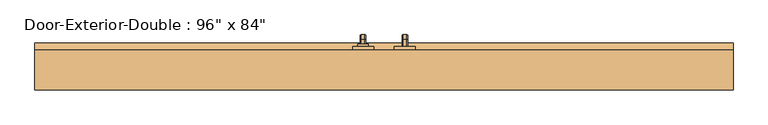
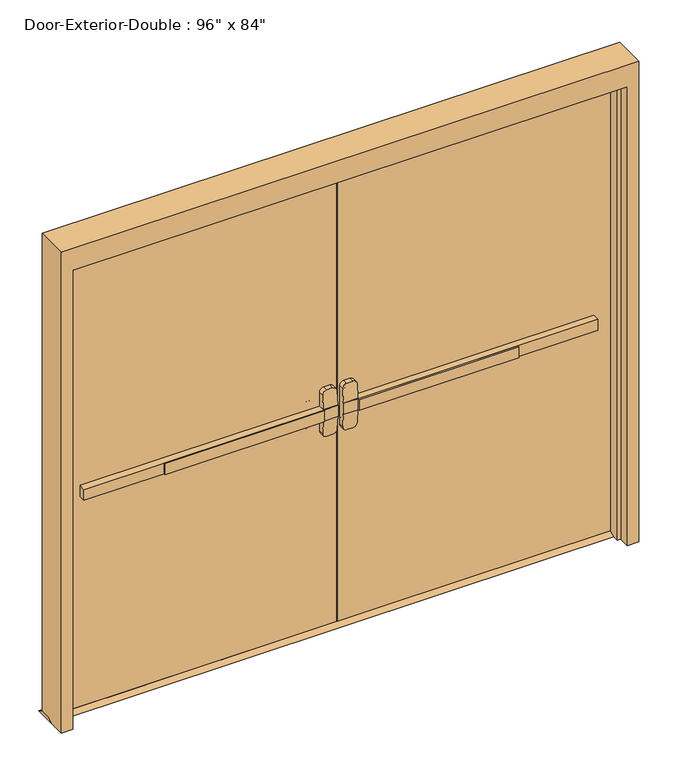
"""IFC4 building model written with IfcOpenShell, lengths in millimetres: door geometry."""

from ifc_helpers import new_model, si_unit, point, frame, frame_2d, origin, place, context, project, spatial, polyline, circle_curve, ellipse_curve, trimmed, segment, composite_curve, outline, extrude, faceted_brep, source, transform, mapped, element, save
from ifc_brep_helpers import plane_surface, cylinder_surface, revolved_surface, advanced_brep


def door_9521ecb0(model_context):
    return source(origin(), model_context, "Body", "SolidModel", [
        extrude(outline(polyline([(-778.9333333, 0.0), (-778.9333333, 6.35), (-76.2, 6.35), (-76.2, 0.0), (-778.9333333, 0.0)])), frame((0.0, 0.0, 990.6), z_axis=(0.0, 0.0, 1.0), x_axis=(1.0, 0.0, 0.0)), (0.0, 0.0, 1.0), 50.8),
        advanced_brep(
        [(-12.7, 6.35, 1041.4), (-76.2, 6.35, 1041.4), (-1130.3, 6.35, 1041.4), (-1130.3, 6.35, 990.6), (-76.2, 6.35, 990.6), (-12.7, 6.35, 990.6), (-1130.3, 38.1, 1041.4), (-76.2, 38.1, 1041.4), (-76.2, 38.1, 1104.9), (-57.15, 38.1, 1123.95), (-31.75, 38.1, 1123.95), (-12.7, 38.1, 1104.9), (-12.7, 38.1, 927.1), (-31.75, 38.1, 908.05), (-57.15, 38.1, 908.05), (-76.2, 38.1, 927.1), (-76.2, 38.1, 990.6), (-1130.3, 38.1, 990.6), (-12.7, 9.5252467, 1041.4), (-76.2, 9.5252467, 1041.4), (-12.7, 9.5252467, 990.6), (-12.7, 14.5354269, 927.1), (-12.7, 14.5354269, 1104.9), (-76.2, 9.5252467, 990.6), (-76.2, 14.5354269, 1104.9), (-76.2, 14.5354269, 927.1), (-57.15, 16.038481, 1123.95), (-31.75, 16.038481, 1123.95), (-31.75, 16.038481, 908.05), (-57.15, 16.038481, 908.05)],
        [
            (0, 1),
            (1, 2),
            (2, 3),
            (3, 4),
            (4, 5),
            (5, 0),
            (6, 7),
            (7, 8),
            (8, 9, circle_curve(frame((-57.15, 38.1, 1104.9), z_axis=(0.0, 1.0, 0.0), x_axis=(-1.0, 0.0, 0.0)), 19.05)),
            (9, 10),
            (10, 11, circle_curve(frame((-31.75, 38.1, 1104.9), z_axis=(0.0, 1.0, 0.0), x_axis=(-1.0, 0.0, 0.0)), 19.05)),
            (11, 12),
            (12, 13, circle_curve(frame((-31.75, 38.1, 927.1), z_axis=(0.0, 1.0, 0.0), x_axis=(-1.0, 0.0, 0.0)), 19.05)),
            (13, 14),
            (14, 15, circle_curve(frame((-57.15, 38.1, 927.1), z_axis=(0.0, 1.0, 0.0), x_axis=(-1.0, 0.0, 0.0)), 19.05)),
            (15, 16),
            (16, 17),
            (17, 6),
            (0, 18),
            (18, 19),
            (19, 7),
            (6, 2),
            (5, 20),
            (20, 21),
            (21, 12),
            (11, 22),
            (22, 18),
            (16, 23),
            (23, 20),
            (3, 17),
            (19, 24),
            (24, 8),
            (15, 25),
            (25, 23),
            (9, 26),
            (26, 27),
            (27, 10),
            (13, 28),
            (28, 29),
            (29, 14),
            (29, 25, ellipse_curve(frame((-57.15, 14.5354269, 927.1), z_axis=(0.0, 0.9969018152893365, 0.07865602756830282), x_axis=(0.0, -0.07865602756830208, 0.9969018152893365)), 19.1092038, 19.05)),
            (24, 26, ellipse_curve(frame((-57.15, 14.5354269, 1104.9), z_axis=(0.0, 0.9969018152893376, -0.07865602756828934), x_axis=(0.0, -0.078656027568288, -0.9969018152893377)), 19.1092038, 19.05)),
            (27, 22, ellipse_curve(frame((-31.75, 14.5354269, 1104.9), z_axis=(0.0, 0.9969018152893376, -0.07865602756828934), x_axis=(0.0, -0.078656027568288, -0.9969018152893377)), 19.1092038, 19.05)),
            (21, 28, ellipse_curve(frame((-31.75, 14.5354269, 927.1), z_axis=(0.0, 0.9969018152893365, 0.07865602756830282), x_axis=(0.0, -0.07865602756830208, 0.9969018152893365)), 19.1092038, 19.05)),
        ],
        [
            plane_surface(frame((-12.7, 6.35, 1041.4), z_axis=(0.0, -1.0, 0.0), x_axis=(1.0, 0.0, 0.0))),
            plane_surface(frame((-12.7, 38.1, 1041.4), z_axis=(0.0, 1.0, 0.0), x_axis=(-1.0, 0.0, 0.0))),
            plane_surface(frame((-1130.3, 6.35, 1041.4), z_axis=(0.0, 0.0, 1.0), x_axis=(0.0, 1.0, 0.0))),
            plane_surface(frame((-12.7, 6.35, 1041.4), z_axis=(1.0, 0.0, 0.0), x_axis=(0.0, 1.0, 0.0))),
            plane_surface(frame((-12.7, 6.35, 990.6), z_axis=(0.0, 0.0, -1.0), x_axis=(0.0, 1.0, 0.0))),
            plane_surface(frame((-1130.3, 6.35, 990.6), z_axis=(-1.0, 0.0, 0.0), x_axis=(0.0, 1.0, 0.0))),
            plane_surface(frame((-76.2, 9.5252467, 927.1), z_axis=(-1.0, 0.0, 0.0), x_axis=(0.0, 1.0, 0.0))),
            plane_surface(frame((-57.15, 9.5252467, 1123.95), z_axis=(0.0, 0.0, 1.0), x_axis=(0.0, 1.0, 0.0))),
            plane_surface(frame((-31.75, 9.5252467, 908.05), z_axis=(0.0, 0.0, -1.0), x_axis=(0.0, 1.0, 0.0))),
            cylinder_surface(frame((-57.15, 38.1, 927.1), z_axis=(0.0, -1.0, 0.0), x_axis=(-1.0, 0.0, 0.0)), 19.05),
            cylinder_surface(frame((-57.15, 38.1, 1104.9), z_axis=(0.0, -1.0, 0.0), x_axis=(-1.0, 0.0, 0.0)), 19.05),
            cylinder_surface(frame((-31.75, 38.1, 1104.9), z_axis=(0.0, -1.0, 0.0), x_axis=(-1.0, 0.0, 0.0)), 19.05),
            cylinder_surface(frame((-31.75, 38.1, 927.1), z_axis=(0.0, -1.0, 0.0), x_axis=(-1.0, 0.0, 0.0)), 19.05),
            plane_surface(frame((-76.2, 9.5252467, 1041.4), z_axis=(0.0, -0.9969018152893376, 0.07865602756828934), x_axis=(1.0, 0.0, 0.0))),
            plane_surface(frame((-76.2, 16.038481, 908.05), z_axis=(0.0, -0.9969018152893365, -0.07865602756830282), x_axis=(1.0, 0.0, 0.0))),
        ],
        [
            (0, [[1, 2, 3, 4, 5, 6]]),
            (1, [[7, 8, 9, 10, 11, 12, 13, 14, 15, 16, 17, 18]]),
            (2, [[-2, -1, 19, 20, 21, -7, 22]]),
            (3, [[23, 24, 25, -12, 26, 27, -19, -6]]),
            (4, [[-17, 28, 29, -23, -5, -4, 30]]),
            (5, [[-22, -18, -30, -3]]),
            (6, [[-21, 31, 32, -8]]),
            (6, [[33, 34, -28, -16]]),
            (7, [[35, 36, 37, -10]]),
            (8, [[38, 39, 40, -14]]),
            (9, [[-40, 41, -33, -15]]),
            (10, [[-32, 42, -35, -9]]),
            (11, [[-37, 43, -26, -11]]),
            (12, [[-25, 44, -38, -13]]),
            (13, [[-27, -43, -36, -42, -31, -20]]),
            (14, [[-29, -34, -41, -39, -44, -24]]),
        ],
    ),
        extrude(outline(polyline([(82.55, 12.7), (107.95, 0.0), (12.7, 0.0), (38.1, 12.7), (82.55, 12.7)])), frame((-1270.0, 0.0, 0.0), z_axis=(1.0, 0.0, 0.0), x_axis=(0.0, 1.0, 0.0)), (0.0, 0.0, 1.0), 2540.0),
        extrude(outline(polyline([(778.9333333, 0.0), (76.2, 0.0), (76.2, 6.35), (778.9333333, 6.35), (778.9333333, 0.0)])), frame((0.0, 0.0, 990.6), z_axis=(0.0, 0.0, 1.0), x_axis=(1.0, 0.0, 0.0)), (0.0, 0.0, 1.0), 50.8),
        advanced_brep(
        [(12.7, 6.35, 1041.4), (12.7, 6.35, 990.6), (76.2, 6.35, 990.6), (1130.3, 6.35, 990.6), (1130.3, 6.35, 1041.4), (76.2, 6.35, 1041.4), (1130.3, 38.1, 1041.4), (1130.3, 38.1, 990.6), (76.2, 38.1, 990.6), (76.2, 38.1, 927.1), (57.15, 38.1, 908.05), (31.75, 38.1, 908.05), (12.7, 38.1, 927.1), (12.7, 38.1, 1104.9), (31.75, 38.1, 1123.95), (57.15, 38.1, 1123.95), (76.2, 38.1, 1104.9), (76.2, 38.1, 1041.4), (76.2, 9.5252467, 1041.4), (12.7, 9.5252467, 1041.4), (12.7, 14.5354269, 1104.9), (12.7, 14.5354269, 927.1), (12.7, 9.5252467, 990.6), (76.2, 9.5252467, 990.6), (76.2, 14.5354269, 927.1), (76.2, 14.5354269, 1104.9), (31.75, 16.038481, 1123.95), (57.15, 16.038481, 1123.95), (57.15, 16.038481, 908.05), (31.75, 16.038481, 908.05)],
        [
            (0, 1),
            (1, 2),
            (2, 3),
            (3, 4),
            (4, 5),
            (5, 0),
            (6, 7),
            (7, 8),
            (8, 9),
            (9, 10, circle_curve(frame((57.15, 38.1, 927.1), z_axis=(0.0, 1.0, 0.0), x_axis=(1.0, 0.0, 0.0)), 19.05)),
            (10, 11),
            (11, 12, circle_curve(frame((31.75, 38.1, 927.1), z_axis=(0.0, 1.0, 0.0), x_axis=(1.0, 0.0, 0.0)), 19.05)),
            (12, 13),
            (13, 14, circle_curve(frame((31.75, 38.1, 1104.9), z_axis=(0.0, 1.0, 0.0), x_axis=(1.0, 0.0, 0.0)), 19.05)),
            (14, 15),
            (15, 16, circle_curve(frame((57.15, 38.1, 1104.9), z_axis=(0.0, 1.0, 0.0), x_axis=(1.0, 0.0, 0.0)), 19.05)),
            (16, 17),
            (17, 6),
            (4, 6),
            (17, 18),
            (18, 19),
            (19, 0),
            (19, 20),
            (20, 13),
            (12, 21),
            (21, 22),
            (22, 1),
            (7, 3),
            (22, 23),
            (23, 8),
            (23, 24),
            (24, 9),
            (16, 25),
            (25, 18),
            (14, 26),
            (26, 27),
            (27, 15),
            (10, 28),
            (28, 29),
            (29, 11),
            (24, 28, ellipse_curve(frame((57.15, 14.5354269, 927.1), z_axis=(0.0, 0.9969018152893365, 0.07865602756830282), x_axis=(0.0, -0.07865602756830208, 0.9969018152893365)), 19.1092038, 19.05)),
            (27, 25, ellipse_curve(frame((57.15, 14.5354269, 1104.9), z_axis=(0.0, 0.9969018152893376, -0.07865602756828934), x_axis=(0.0, -0.078656027568288, -0.9969018152893377)), 19.1092038, 19.05)),
            (20, 26, ellipse_curve(frame((31.75, 14.5354269, 1104.9), z_axis=(0.0, 0.9969018152893376, -0.07865602756828934), x_axis=(0.0, -0.078656027568288, -0.9969018152893377)), 19.1092038, 19.05)),
            (29, 21, ellipse_curve(frame((31.75, 14.5354269, 927.1), z_axis=(0.0, 0.9969018152893365, 0.07865602756830282), x_axis=(0.0, -0.07865602756830208, 0.9969018152893365)), 19.1092038, 19.05)),
        ],
        [
            plane_surface(frame((12.7, 6.35, 1041.4), z_axis=(0.0, -1.0, 0.0), x_axis=(-1.0, 0.0, 0.0))),
            plane_surface(frame((12.7, 38.1, 1041.4), z_axis=(0.0, 1.0, 0.0), x_axis=(1.0, 0.0, 0.0))),
            plane_surface(frame((1130.3, 6.35, 1041.4), z_axis=(0.0, 0.0, 1.0), x_axis=(0.0, 1.0, 0.0))),
            plane_surface(frame((12.7, 6.35, 1041.4), z_axis=(-1.0, 0.0, 0.0), x_axis=(0.0, 1.0, 0.0))),
            plane_surface(frame((12.7, 6.35, 990.6), z_axis=(0.0, 0.0, -1.0), x_axis=(0.0, 1.0, 0.0))),
            plane_surface(frame((1130.3, 6.35, 990.6), z_axis=(1.0, 0.0, 0.0), x_axis=(0.0, 1.0, 0.0))),
            plane_surface(frame((76.2, 9.5252467, 927.1), z_axis=(1.0, 0.0, 0.0), x_axis=(0.0, 1.0, 0.0))),
            plane_surface(frame((57.15, 9.5252467, 1123.95), z_axis=(0.0, 0.0, 1.0), x_axis=(0.0, 1.0, 0.0))),
            plane_surface(frame((31.75, 9.5252467, 908.05), z_axis=(0.0, 0.0, -1.0), x_axis=(0.0, 1.0, 0.0))),
            cylinder_surface(frame((57.15, 38.1, 927.1), z_axis=(0.0, -1.0, 0.0), x_axis=(1.0, 0.0, 0.0)), 19.05),
            cylinder_surface(frame((57.15, 38.1, 1104.9), z_axis=(0.0, -1.0, 0.0), x_axis=(1.0, 0.0, 0.0)), 19.05),
            cylinder_surface(frame((31.75, 38.1, 1104.9), z_axis=(0.0, -1.0, 0.0), x_axis=(1.0, 0.0, 0.0)), 19.05),
            cylinder_surface(frame((31.75, 38.1, 927.1), z_axis=(0.0, -1.0, 0.0), x_axis=(1.0, 0.0, 0.0)), 19.05),
            plane_surface(frame((76.2, 9.5252467, 1041.4), z_axis=(0.0, -0.9969018152893376, 0.07865602756828934), x_axis=(-1.0, 0.0, 0.0))),
            plane_surface(frame((76.2, 16.038481, 908.05), z_axis=(0.0, -0.9969018152893365, -0.07865602756830282), x_axis=(-1.0, 0.0, 0.0))),
        ],
        [
            (0, [[1, 2, 3, 4, 5, 6]]),
            (1, [[7, 8, 9, 10, 11, 12, 13, 14, 15, 16, 17, 18]]),
            (2, [[19, -18, 20, 21, 22, -6, -5]]),
            (3, [[-1, -22, 23, 24, -13, 25, 26, 27]]),
            (4, [[28, -3, -2, -27, 29, 30, -8]]),
            (5, [[-4, -28, -7, -19]]),
            (6, [[-9, -30, 31, 32]]),
            (6, [[-17, 33, 34, -20]]),
            (7, [[-15, 35, 36, 37]]),
            (8, [[-11, 38, 39, 40]]),
            (9, [[-10, -32, 41, -38]]),
            (10, [[-16, -37, 42, -33]]),
            (11, [[-14, -24, 43, -35]]),
            (12, [[-12, -40, 44, -25]]),
            (13, [[-21, -34, -42, -36, -43, -23]]),
            (14, [[-26, -44, -39, -41, -31, -29]]),
        ],
    ),
        advanced_brep(
        [(66.2, 95.25, 1017.190625), (66.2, 95.25, 1014.809375), (69.771875, 95.25, 1011.2375), (82.6284594, 95.25, 1011.2375), (86.2, 95.25, 1014.8090406), (86.2, 95.25, 1017.190625), (82.628125, 95.25, 1020.7625), (69.771875, 95.25, 1020.7625), (66.2, 95.25, 887.809375), (69.771875, 95.25, 884.2375), (82.628125, 95.25, 884.2375), (86.2, 95.25, 887.809375), (86.2, 95.25, 890.1909594), (82.6284594, 95.25, 893.7625), (69.771875, 95.25, 893.7625), (66.2, 95.25, 890.190625), (66.2, 120.65, 1017.190625), (66.2, 134.540625, 1003.3), (66.2, 134.540625, 901.7), (66.2, 120.65, 887.809375), (66.2, 120.65, 890.190625), (66.2, 132.159375, 901.7), (66.2, 132.159375, 1003.3), (66.2, 120.65, 1014.809375), (69.771875, 120.65, 1011.2375), (82.6284594, 120.65, 1011.2375), (86.2, 120.65, 1014.8090406), (86.2, 132.1590406, 1003.3), (86.2, 132.1590406, 901.7), (86.2, 120.65, 890.1909594), (86.2, 120.65, 887.809375), (86.2, 134.540625, 901.7), (86.2, 134.540625, 1003.3), (86.2, 120.65, 1017.190625), (82.628125, 120.65, 1020.7625), (69.771875, 120.65, 1020.7625), (69.771875, 128.5875, 1003.3), (82.6284594, 128.5875, 1003.3), (82.628125, 138.1125, 1003.3), (69.771875, 138.1125, 1003.3), (69.771875, 128.5875, 901.7), (82.6284594, 128.5875, 901.7), (82.628125, 138.1125, 901.7), (69.771875, 138.1125, 901.7), (69.771875, 120.65, 893.7625), (82.6284594, 120.65, 893.7625), (82.628125, 120.65, 884.2375), (69.771875, 120.65, 884.2375)],
        [
            (0, 1),
            (1, 2, circle_curve(frame((69.771875, 95.25, 1014.809375), z_axis=(0.0, -1.0, 0.0), x_axis=(0.0, 0.0, 1.0)), 3.571875)),
            (2, 3),
            (3, 4, circle_curve(frame((82.6284594, 95.25, 1014.8090406), z_axis=(0.0, -1.0, 0.0), x_axis=(0.0, 0.0, 1.0)), 3.5715406)),
            (4, 5),
            (5, 6, circle_curve(frame((82.628125, 95.25, 1017.190625), z_axis=(0.0, -1.0, 0.0), x_axis=(0.0, 0.0, 1.0)), 3.571875)),
            (6, 7),
            (7, 0, circle_curve(frame((69.771875, 95.25, 1017.190625), z_axis=(0.0, -1.0, 0.0), x_axis=(0.0, 0.0, 1.0)), 3.571875)),
            (8, 9, circle_curve(frame((69.771875, 95.25, 887.809375), z_axis=(0.0, -1.0, 0.0), x_axis=(0.0, 0.0, -1.0)), 3.571875)),
            (9, 10),
            (10, 11, circle_curve(frame((82.628125, 95.25, 887.809375), z_axis=(0.0, -1.0, 0.0), x_axis=(0.0, 0.0, -1.0)), 3.571875)),
            (11, 12),
            (12, 13, circle_curve(frame((82.6284594, 95.25, 890.1909594), z_axis=(0.0, -1.0, 0.0), x_axis=(0.0, 0.0, -1.0)), 3.5715406)),
            (13, 14),
            (14, 15, circle_curve(frame((69.771875, 95.25, 890.190625), z_axis=(0.0, -1.0, 0.0), x_axis=(0.0, 0.0, -1.0)), 3.571875)),
            (15, 8),
            (0, 16),
            (16, 17, circle_curve(frame((66.2, 120.65, 1003.3), z_axis=(-1.0, 0.0, 0.0), x_axis=(0.0, 0.0, 1.0)), 13.890625)),
            (17, 18),
            (18, 19, circle_curve(frame((66.2, 120.65, 901.7), z_axis=(-1.0, 0.0, 0.0), x_axis=(0.0, 1.0, 0.0)), 13.890625)),
            (19, 8),
            (15, 20),
            (20, 21, circle_curve(frame((66.2, 120.65, 901.7), z_axis=(1.0, 0.0, 0.0), x_axis=(0.0, 1.0, 0.0)), 11.509375)),
            (21, 22),
            (22, 23, circle_curve(frame((66.2, 120.65, 1003.3), z_axis=(1.0, 0.0, 0.0), x_axis=(0.0, 0.0, 1.0)), 11.509375)),
            (23, 1),
            (23, 24, circle_curve(frame((69.771875, 120.65, 1014.809375), z_axis=(0.0, -1.0, 0.0), x_axis=(0.0, 0.0, 1.0)), 3.571875)),
            (24, 2),
            (24, 25),
            (25, 3),
            (25, 26, circle_curve(frame((82.6284594, 120.65, 1014.8090406), z_axis=(0.0, -1.0, 0.0), x_axis=(0.0, 0.0, 1.0)), 3.5715406)),
            (26, 4),
            (26, 27, circle_curve(frame((86.2, 120.65, 1003.3), z_axis=(-1.0, 0.0, 0.0), x_axis=(0.0, 0.0, 1.0)), 11.5090406)),
            (27, 28),
            (28, 29, circle_curve(frame((86.2, 120.65, 901.7), z_axis=(-1.0, 0.0, 0.0), x_axis=(0.0, 1.0, 0.0)), 11.5090406)),
            (29, 12),
            (11, 30),
            (30, 31, circle_curve(frame((86.2, 120.65, 901.7), z_axis=(1.0, 0.0, 0.0), x_axis=(0.0, 1.0, 0.0)), 13.890625)),
            (31, 32),
            (32, 33, circle_curve(frame((86.2, 120.65, 1003.3), z_axis=(1.0, 0.0, 0.0), x_axis=(0.0, 0.0, 1.0)), 13.890625)),
            (33, 5),
            (33, 34, circle_curve(frame((82.628125, 120.65, 1017.190625), z_axis=(0.0, -1.0, 0.0), x_axis=(0.0, 0.0, 1.0)), 3.571875)),
            (34, 6),
            (34, 35),
            (35, 7),
            (35, 16, circle_curve(frame((69.771875, 120.65, 1017.190625), z_axis=(0.0, -1.0, 0.0), x_axis=(0.0, 0.0, 1.0)), 3.571875)),
            (36, 24, circle_curve(frame((69.771875, 120.65, 1003.3), z_axis=(1.0, 0.0, 0.0), x_axis=(0.0, 0.0, 1.0)), 7.9375)),
            (22, 36, circle_curve(frame((69.771875, 132.159375, 1003.3), z_axis=(0.0, 0.0, 1.0), x_axis=(0.0, 1.0, 0.0)), 3.571875)),
            (37, 25, circle_curve(frame((82.6284594, 120.65, 1003.3), z_axis=(1.0, 0.0, 0.0), x_axis=(0.0, 0.0, 1.0)), 7.9375)),
            (36, 37),
            (37, 27, circle_curve(frame((82.6284594, 132.1590406, 1003.3), z_axis=(0.0, 0.0, 1.0), x_axis=(0.0, 1.0, 0.0)), 3.5715406)),
            (38, 34, circle_curve(frame((82.628125, 120.65, 1003.3), z_axis=(1.0, 0.0, 0.0), x_axis=(0.0, 0.0, 1.0)), 17.4625)),
            (32, 38, circle_curve(frame((82.628125, 134.540625, 1003.3), z_axis=(0.0, 0.0, 1.0), x_axis=(0.0, 1.0, 0.0)), 3.571875)),
            (39, 35, circle_curve(frame((69.771875, 120.65, 1003.3), z_axis=(1.0, 0.0, 0.0), x_axis=(0.0, 0.0, 1.0)), 17.4625)),
            (38, 39),
            (39, 17, circle_curve(frame((69.771875, 134.540625, 1003.3), z_axis=(0.0, 0.0, 1.0), x_axis=(0.0, 1.0, 0.0)), 3.571875)),
            (21, 40, circle_curve(frame((69.771875, 132.159375, 901.7), z_axis=(0.0, 0.0, 1.0), x_axis=(0.0, 1.0, 0.0)), 3.571875)),
            (40, 36),
            (40, 41),
            (41, 37),
            (41, 28, circle_curve(frame((82.6284594, 132.1590406, 901.7), z_axis=(0.0, 0.0, 1.0), x_axis=(0.0, 1.0, 0.0)), 3.5715406)),
            (31, 42, circle_curve(frame((82.628125, 134.540625, 901.7), z_axis=(0.0, 0.0, 1.0), x_axis=(0.0, 1.0, 0.0)), 3.571875)),
            (42, 38),
            (42, 43),
            (43, 39),
            (43, 18, circle_curve(frame((69.771875, 134.540625, 901.7), z_axis=(0.0, 0.0, 1.0), x_axis=(0.0, 1.0, 0.0)), 3.571875)),
            (44, 40, circle_curve(frame((69.771875, 120.65, 901.7), z_axis=(1.0, 0.0, 0.0), x_axis=(0.0, 1.0, 0.0)), 7.9375)),
            (20, 44, circle_curve(frame((69.771875, 120.65, 890.190625), z_axis=(0.0, 1.0, 0.0), x_axis=(0.0, 0.0, -1.0)), 3.571875)),
            (45, 41, circle_curve(frame((82.6284594, 120.65, 901.7), z_axis=(1.0, 0.0, 0.0), x_axis=(0.0, 1.0, 0.0)), 7.9375)),
            (44, 45),
            (45, 29, circle_curve(frame((82.6284594, 120.65, 890.1909594), z_axis=(0.0, 1.0, 0.0), x_axis=(0.0, 0.0, -1.0)), 3.5715406)),
            (46, 42, circle_curve(frame((82.628125, 120.65, 901.7), z_axis=(1.0, 0.0, 0.0), x_axis=(0.0, 1.0, 0.0)), 17.4625)),
            (30, 46, circle_curve(frame((82.628125, 120.65, 887.809375), z_axis=(0.0, 1.0, 0.0), x_axis=(0.0, 0.0, -1.0)), 3.571875)),
            (47, 43, circle_curve(frame((69.771875, 120.65, 901.7), z_axis=(1.0, 0.0, 0.0), x_axis=(0.0, 1.0, 0.0)), 17.4625)),
            (46, 47),
            (47, 19, circle_curve(frame((69.771875, 120.65, 887.809375), z_axis=(0.0, 1.0, 0.0), x_axis=(0.0, 0.0, -1.0)), 3.571875)),
            (14, 44),
            (13, 45),
            (10, 46),
            (9, 47),
        ],
        [
            plane_surface(frame((76.2, 95.25, 1016.0), z_axis=(0.0, -1.0, 0.0), x_axis=(1.0, 0.0, 0.0))),
            plane_surface(frame((76.2, 95.25, 889.0), z_axis=(0.0, -1.0, 0.0), x_axis=(1.0, 0.0, 0.0))),
            plane_surface(frame((66.2, 95.25, 1017.190625), z_axis=(-1.0, 0.0, 0.0), x_axis=(0.0, 1.0, 0.0))),
            cylinder_surface(frame((69.771875, 95.25, 1014.809375), z_axis=(0.0, -1.0, 0.0), x_axis=(0.0, 0.0, 1.0)), 3.571875),
            plane_surface(frame((69.771875, 95.25, 1011.2375), z_axis=(0.0, 0.0, -1.0), x_axis=(0.0, 1.0, 0.0))),
            cylinder_surface(frame((82.6284594, 95.25, 1014.8090406), z_axis=(0.0, -1.0, 0.0), x_axis=(0.0, 0.0, 1.0)), 3.5715406),
            plane_surface(frame((86.2, 95.25, 1014.8090406), z_axis=(1.0, 0.0, 0.0), x_axis=(0.0, 1.0, 0.0))),
            cylinder_surface(frame((82.628125, 95.25, 1017.190625), z_axis=(0.0, -1.0, 0.0), x_axis=(0.0, 0.0, 1.0)), 3.571875),
            plane_surface(frame((82.628125, 95.25, 1020.7625), z_axis=(0.0, 0.0, 1.0), x_axis=(0.0, 1.0, 0.0))),
            cylinder_surface(frame((69.771875, 95.25, 1017.190625), z_axis=(0.0, -1.0, 0.0), x_axis=(0.0, 0.0, 1.0)), 3.571875),
            revolved_surface(trimmed(ellipse_curve(frame((69.771875, 120.65, 1014.809375), z_axis=(0.0, -1.0, 0.0), x_axis=(0.0, 0.0, 1.0)), 3.571875, 3.571875), [point((66.2, 120.65, 1014.809375))], [point((69.771875, 120.65, 1011.2375))], True, "CARTESIAN"), (76.2, 120.65, 1003.3), (-1.0, 0.0, 0.0)),
            revolved_surface(polyline([(69.771875, 120.65, 1011.2375), (82.6284594, 120.65, 1011.2375)]), (76.2, 120.65, 1003.3), (-1.0, 0.0, 0.0)),
            revolved_surface(trimmed(ellipse_curve(frame((82.6284594, 120.65, 1014.8090406), z_axis=(0.0, -1.0, 0.0), x_axis=(0.0, 0.0, 1.0)), 3.5715406, 3.5715406), [point((82.6284594, 120.65, 1011.2375))], [point((86.2, 120.65, 1014.8090406))], True, "CARTESIAN"), (76.2, 120.65, 1003.3), (-1.0, 0.0, 0.0)),
            revolved_surface(trimmed(ellipse_curve(frame((82.628125, 120.65, 1017.190625), z_axis=(0.0, -1.0, 0.0), x_axis=(0.0, 0.0, 1.0)), 3.571875, 3.571875), [point((86.2, 120.65, 1017.190625))], [point((82.628125, 120.65, 1020.7625))], True, "CARTESIAN"), (76.2, 120.65, 1003.3), (-1.0, 0.0, 0.0)),
            cylinder_surface(frame((76.2, 120.65, 1003.3), z_axis=(-1.0, 0.0, 0.0), x_axis=(0.0, 0.0, 1.0)), 17.4625),
            revolved_surface(trimmed(ellipse_curve(frame((69.771875, 120.65, 1017.190625), z_axis=(0.0, -1.0, 0.0), x_axis=(0.0, 0.0, 1.0)), 3.571875, 3.571875), [point((69.771875, 120.65, 1020.7625))], [point((66.2, 120.65, 1017.190625))], True, "CARTESIAN"), (76.2, 120.65, 1003.3), (-1.0, 0.0, 0.0)),
            cylinder_surface(frame((69.771875, 132.159375, 1003.3), z_axis=(0.0, 0.0, 1.0), x_axis=(0.0, 1.0, 0.0)), 3.571875),
            plane_surface(frame((69.771875, 128.5875, 1003.3), z_axis=(0.0, -1.0, 0.0), x_axis=(0.0, 0.0, -1.0))),
            cylinder_surface(frame((82.6284594, 132.1590406, 1003.3), z_axis=(0.0, 0.0, 1.0), x_axis=(0.0, 1.0, 0.0)), 3.5715406),
            cylinder_surface(frame((82.628125, 134.540625, 1003.3), z_axis=(0.0, 0.0, 1.0), x_axis=(0.0, 1.0, 0.0)), 3.571875),
            plane_surface(frame((82.628125, 138.1125, 1003.3), z_axis=(0.0, 1.0, 0.0), x_axis=(0.0, 0.0, -1.0))),
            cylinder_surface(frame((69.771875, 134.540625, 1003.3), z_axis=(0.0, 0.0, 1.0), x_axis=(0.0, 1.0, 0.0)), 3.571875),
            revolved_surface(trimmed(ellipse_curve(frame((69.771875, 132.159375, 901.7), z_axis=(0.0, 0.0, 1.0), x_axis=(0.0, 1.0, 0.0)), 3.571875, 3.571875), [point((66.2, 132.159375, 901.7))], [point((69.771875, 128.5875, 901.7))], True, "CARTESIAN"), (76.2, 120.65, 901.7), (-1.0, 0.0, 0.0)),
            revolved_surface(polyline([(69.771875, 128.5875, 901.7), (82.6284594, 128.5875, 901.7)]), (76.2, 120.65, 901.7), (-1.0, 0.0, 0.0)),
            revolved_surface(trimmed(ellipse_curve(frame((82.6284594, 132.1590406, 901.7), z_axis=(0.0, 0.0, 1.0), x_axis=(0.0, 1.0, 0.0)), 3.5715406, 3.5715406), [point((82.6284594, 128.5875, 901.7))], [point((86.2, 132.1590406, 901.7))], True, "CARTESIAN"), (76.2, 120.65, 901.7), (-1.0, 0.0, 0.0)),
            revolved_surface(trimmed(ellipse_curve(frame((82.628125, 134.540625, 901.7), z_axis=(0.0, 0.0, 1.0), x_axis=(0.0, 1.0, 0.0)), 3.571875, 3.571875), [point((86.2, 134.540625, 901.7))], [point((82.628125, 138.1125, 901.7))], True, "CARTESIAN"), (76.2, 120.65, 901.7), (-1.0, 0.0, 0.0)),
            cylinder_surface(frame((76.2, 120.65, 901.7), z_axis=(-1.0, 0.0, 0.0), x_axis=(0.0, 1.0, 0.0)), 17.4625),
            revolved_surface(trimmed(ellipse_curve(frame((69.771875, 134.540625, 901.7), z_axis=(0.0, 0.0, 1.0), x_axis=(0.0, 1.0, 0.0)), 3.571875, 3.571875), [point((69.771875, 138.1125, 901.7))], [point((66.2, 134.540625, 901.7))], True, "CARTESIAN"), (76.2, 120.65, 901.7), (-1.0, 0.0, 0.0)),
            cylinder_surface(frame((69.771875, 120.65, 890.190625), z_axis=(0.0, 1.0, 0.0), x_axis=(0.0, 0.0, -1.0)), 3.571875),
            plane_surface(frame((69.771875, 120.65, 893.7625), z_axis=(0.0, 0.0, 1.0), x_axis=(0.0, -1.0, 0.0))),
            cylinder_surface(frame((82.6284594, 120.65, 890.1909594), z_axis=(0.0, 1.0, 0.0), x_axis=(0.0, 0.0, -1.0)), 3.5715406),
            cylinder_surface(frame((82.628125, 120.65, 887.809375), z_axis=(0.0, 1.0, 0.0), x_axis=(0.0, 0.0, -1.0)), 3.571875),
            plane_surface(frame((82.628125, 120.65, 884.2375), z_axis=(0.0, 0.0, -1.0), x_axis=(0.0, -1.0, 0.0))),
            cylinder_surface(frame((69.771875, 120.65, 887.809375), z_axis=(0.0, 1.0, 0.0), x_axis=(0.0, 0.0, -1.0)), 3.571875),
        ],
        [
            (0, [[1, 2, 3, 4, 5, 6, 7, 8]]),
            (1, [[9, 10, 11, 12, 13, 14, 15, 16]]),
            (2, [[-1, 17, 18, 19, 20, 21, -16, 22, 23, 24, 25, 26]]),
            (3, [[-2, -26, 27, 28]]),
            (4, [[-3, -28, 29, 30]]),
            (5, [[-4, -30, 31, 32]]),
            (6, [[-5, -32, 33, 34, 35, 36, -12, 37, 38, 39, 40, 41]]),
            (7, [[-6, -41, 42, 43]]),
            (8, [[-7, -43, 44, 45]]),
            (9, [[-8, -45, 46, -17]]),
            (10, [[47, -27, -25, 48]]),
            (11, [[49, -29, -47, 50]]),
            (12, [[-33, -31, -49, 51]]),
            (13, [[52, -42, -40, 53]]),
            (14, [[54, -44, -52, 55]]),
            (15, [[-18, -46, -54, 56]]),
            (16, [[-48, -24, 57, 58]]),
            (17, [[-50, -58, 59, 60]]),
            (18, [[-51, -60, 61, -34]]),
            (19, [[-53, -39, 62, 63]]),
            (20, [[-55, -63, 64, 65]]),
            (21, [[-56, -65, 66, -19]]),
            (22, [[67, -57, -23, 68]]),
            (23, [[69, -59, -67, 70]]),
            (24, [[-35, -61, -69, 71]]),
            (25, [[72, -62, -38, 73]]),
            (26, [[74, -64, -72, 75]]),
            (27, [[-20, -66, -74, 76]]),
            (28, [[-68, -22, -15, 77]]),
            (29, [[-70, -77, -14, 78]]),
            (30, [[-71, -78, -13, -36]]),
            (31, [[-73, -37, -11, 79]]),
            (32, [[-75, -79, -10, 80]]),
            (33, [[-76, -80, -9, -21]]),
        ],
    ),
        extrude(outline(composite_curve([segment(trimmed(circle_curve(frame_2d((1113.0338574, 76.2)), 89.3016225), [point((1193.8, 114.3))], [point((1193.8, 38.1))], False, "CARTESIAN"), True, "CONTINUOUS"), segment(polyline([(1193.8, 38.1), (838.2, 38.1)]), True, "CONTINUOUS"), segment(trimmed(circle_curve(frame_2d((918.9661426, 76.2)), 89.3016225), [point((838.2, 38.1))], [point((838.2, 114.3))], False, "CARTESIAN"), True, "CONTINUOUS"), segment(polyline([(838.2, 114.3), (1193.8, 114.3)]), True, "CONTINUOUS")], self_intersect=False)), frame((0.0, 82.55, 0.0), z_axis=(0.0, 1.0, 0.0), x_axis=(0.0, 0.0, 1.0)), (0.0, 0.0, 1.0), 12.7),
        advanced_brep(
        [(-86.2, 95.25, 1017.190625), (-86.2, 95.25, 1014.809375), (-82.628125, 95.25, 1011.2375), (-69.7715406, 95.25, 1011.2375), (-66.2, 95.25, 1014.8090406), (-66.2, 95.25, 1017.190625), (-69.771875, 95.25, 1020.7625), (-82.628125, 95.25, 1020.7625), (-86.2, 95.25, 887.809375), (-82.628125, 95.25, 884.2375), (-69.771875, 95.25, 884.2375), (-66.2, 95.25, 887.809375), (-66.2, 95.25, 890.1909594), (-69.7715406, 95.25, 893.7625), (-82.628125, 95.25, 893.7625), (-86.2, 95.25, 890.190625), (-86.2, 120.65, 1017.190625), (-86.2, 134.540625, 1003.3), (-86.2, 134.540625, 901.7), (-86.2, 120.65, 887.809375), (-86.2, 120.65, 890.190625), (-86.2, 132.159375, 901.7), (-86.2, 132.159375, 1003.3), (-86.2, 120.65, 1014.809375), (-82.628125, 120.65, 1011.2375), (-69.7715406, 120.65, 1011.2375), (-66.2, 120.65, 1014.8090406), (-66.2, 132.1590406, 1003.3), (-66.2, 132.1590406, 901.7), (-66.2, 120.65, 890.1909594), (-66.2, 120.65, 887.809375), (-66.2, 134.540625, 901.7), (-66.2, 134.540625, 1003.3), (-66.2, 120.65, 1017.190625), (-69.771875, 120.65, 1020.7625), (-82.628125, 120.65, 1020.7625), (-82.628125, 128.5875, 1003.3), (-69.7715406, 128.5875, 1003.3), (-69.771875, 138.1125, 1003.3), (-82.628125, 138.1125, 1003.3), (-82.628125, 128.5875, 901.7), (-69.7715406, 128.5875, 901.7), (-69.771875, 138.1125, 901.7), (-82.628125, 138.1125, 901.7), (-82.628125, 120.65, 893.7625), (-69.7715406, 120.65, 893.7625), (-69.771875, 120.65, 884.2375), (-82.628125, 120.65, 884.2375)],
        [
            (0, 1),
            (1, 2, circle_curve(frame((-82.628125, 95.25, 1014.809375), z_axis=(0.0, -1.0, 0.0), x_axis=(0.0, 0.0, 1.0)), 3.571875)),
            (2, 3),
            (3, 4, circle_curve(frame((-69.7715406, 95.25, 1014.8090406), z_axis=(0.0, -1.0, 0.0), x_axis=(0.0, 0.0, 1.0)), 3.5715406)),
            (4, 5),
            (5, 6, circle_curve(frame((-69.771875, 95.25, 1017.190625), z_axis=(0.0, -1.0, 0.0), x_axis=(0.0, 0.0, 1.0)), 3.571875)),
            (6, 7),
            (7, 0, circle_curve(frame((-82.628125, 95.25, 1017.190625), z_axis=(0.0, -1.0, 0.0), x_axis=(0.0, 0.0, 1.0)), 3.571875)),
            (8, 9, circle_curve(frame((-82.628125, 95.25, 887.809375), z_axis=(0.0, -1.0, 0.0), x_axis=(0.0, 0.0, -1.0)), 3.571875)),
            (9, 10),
            (10, 11, circle_curve(frame((-69.771875, 95.25, 887.809375), z_axis=(0.0, -1.0, 0.0), x_axis=(0.0, 0.0, -1.0)), 3.571875)),
            (11, 12),
            (12, 13, circle_curve(frame((-69.7715406, 95.25, 890.1909594), z_axis=(0.0, -1.0, 0.0), x_axis=(0.0, 0.0, -1.0)), 3.5715406)),
            (13, 14),
            (14, 15, circle_curve(frame((-82.628125, 95.25, 890.190625), z_axis=(0.0, -1.0, 0.0), x_axis=(0.0, 0.0, -1.0)), 3.571875)),
            (15, 8),
            (0, 16),
            (16, 17, circle_curve(frame((-86.2, 120.65, 1003.3), z_axis=(-1.0, 0.0, 0.0), x_axis=(0.0, 0.0, 1.0)), 13.890625)),
            (17, 18),
            (18, 19, circle_curve(frame((-86.2, 120.65, 901.7), z_axis=(-1.0, 0.0, 0.0), x_axis=(0.0, 1.0, 0.0)), 13.890625)),
            (19, 8),
            (15, 20),
            (20, 21, circle_curve(frame((-86.2, 120.65, 901.7), z_axis=(1.0, 0.0, 0.0), x_axis=(0.0, 1.0, 0.0)), 11.509375)),
            (21, 22),
            (22, 23, circle_curve(frame((-86.2, 120.65, 1003.3), z_axis=(1.0, 0.0, 0.0), x_axis=(0.0, 0.0, 1.0)), 11.509375)),
            (23, 1),
            (23, 24, circle_curve(frame((-82.628125, 120.65, 1014.809375), z_axis=(0.0, -1.0, 0.0), x_axis=(0.0, 0.0, 1.0)), 3.571875)),
            (24, 2),
            (24, 25),
            (25, 3),
            (25, 26, circle_curve(frame((-69.7715406, 120.65, 1014.8090406), z_axis=(0.0, -1.0, 0.0), x_axis=(0.0, 0.0, 1.0)), 3.5715406)),
            (26, 4),
            (26, 27, circle_curve(frame((-66.2, 120.65, 1003.3), z_axis=(-1.0, 0.0, 0.0), x_axis=(0.0, 0.0, 1.0)), 11.5090406)),
            (27, 28),
            (28, 29, circle_curve(frame((-66.2, 120.65, 901.7), z_axis=(-1.0, 0.0, 0.0), x_axis=(0.0, 1.0, 0.0)), 11.5090406)),
            (29, 12),
            (11, 30),
            (30, 31, circle_curve(frame((-66.2, 120.65, 901.7), z_axis=(1.0, 0.0, 0.0), x_axis=(0.0, 1.0, 0.0)), 13.890625)),
            (31, 32),
            (32, 33, circle_curve(frame((-66.2, 120.65, 1003.3), z_axis=(1.0, 0.0, 0.0), x_axis=(0.0, 0.0, 1.0)), 13.890625)),
            (33, 5),
            (33, 34, circle_curve(frame((-69.771875, 120.65, 1017.190625), z_axis=(0.0, -1.0, 0.0), x_axis=(0.0, 0.0, 1.0)), 3.571875)),
            (34, 6),
            (34, 35),
            (35, 7),
            (35, 16, circle_curve(frame((-82.628125, 120.65, 1017.190625), z_axis=(0.0, -1.0, 0.0), x_axis=(0.0, 0.0, 1.0)), 3.571875)),
            (36, 24, circle_curve(frame((-82.628125, 120.65, 1003.3), z_axis=(1.0, 0.0, 0.0), x_axis=(0.0, 0.0, 1.0)), 7.9375)),
            (22, 36, circle_curve(frame((-82.628125, 132.159375, 1003.3), z_axis=(0.0, 0.0, 1.0), x_axis=(0.0, 1.0, 0.0)), 3.571875)),
            (37, 25, circle_curve(frame((-69.7715406, 120.65, 1003.3), z_axis=(1.0, 0.0, 0.0), x_axis=(0.0, 0.0, 1.0)), 7.9375)),
            (36, 37),
            (37, 27, circle_curve(frame((-69.7715406, 132.1590406, 1003.3), z_axis=(0.0, 0.0, 1.0), x_axis=(0.0, 1.0, 0.0)), 3.5715406)),
            (38, 34, circle_curve(frame((-69.771875, 120.65, 1003.3), z_axis=(1.0, 0.0, 0.0), x_axis=(0.0, 0.0, 1.0)), 17.4625)),
            (32, 38, circle_curve(frame((-69.771875, 134.540625, 1003.3), z_axis=(0.0, 0.0, 1.0), x_axis=(0.0, 1.0, 0.0)), 3.571875)),
            (39, 35, circle_curve(frame((-82.628125, 120.65, 1003.3), z_axis=(1.0, 0.0, 0.0), x_axis=(0.0, 0.0, 1.0)), 17.4625)),
            (38, 39),
            (39, 17, circle_curve(frame((-82.628125, 134.540625, 1003.3), z_axis=(0.0, 0.0, 1.0), x_axis=(0.0, 1.0, 0.0)), 3.571875)),
            (21, 40, circle_curve(frame((-82.628125, 132.159375, 901.7), z_axis=(0.0, 0.0, 1.0), x_axis=(0.0, 1.0, 0.0)), 3.571875)),
            (40, 36),
            (40, 41),
            (41, 37),
            (41, 28, circle_curve(frame((-69.7715406, 132.1590406, 901.7), z_axis=(0.0, 0.0, 1.0), x_axis=(0.0, 1.0, 0.0)), 3.5715406)),
            (31, 42, circle_curve(frame((-69.771875, 134.540625, 901.7), z_axis=(0.0, 0.0, 1.0), x_axis=(0.0, 1.0, 0.0)), 3.571875)),
            (42, 38),
            (42, 43),
            (43, 39),
            (43, 18, circle_curve(frame((-82.628125, 134.540625, 901.7), z_axis=(0.0, 0.0, 1.0), x_axis=(0.0, 1.0, 0.0)), 3.571875)),
            (44, 40, circle_curve(frame((-82.628125, 120.65, 901.7), z_axis=(1.0, 0.0, 0.0), x_axis=(0.0, 1.0, 0.0)), 7.9375)),
            (20, 44, circle_curve(frame((-82.628125, 120.65, 890.190625), z_axis=(0.0, 1.0, 0.0), x_axis=(0.0, 0.0, -1.0)), 3.571875)),
            (45, 41, circle_curve(frame((-69.7715406, 120.65, 901.7), z_axis=(1.0, 0.0, 0.0), x_axis=(0.0, 1.0, 0.0)), 7.9375)),
            (44, 45),
            (45, 29, circle_curve(frame((-69.7715406, 120.65, 890.1909594), z_axis=(0.0, 1.0, 0.0), x_axis=(0.0, 0.0, -1.0)), 3.5715406)),
            (46, 42, circle_curve(frame((-69.771875, 120.65, 901.7), z_axis=(1.0, 0.0, 0.0), x_axis=(0.0, 1.0, 0.0)), 17.4625)),
            (30, 46, circle_curve(frame((-69.771875, 120.65, 887.809375), z_axis=(0.0, 1.0, 0.0), x_axis=(0.0, 0.0, -1.0)), 3.571875)),
            (47, 43, circle_curve(frame((-82.628125, 120.65, 901.7), z_axis=(1.0, 0.0, 0.0), x_axis=(0.0, 1.0, 0.0)), 17.4625)),
            (46, 47),
            (47, 19, circle_curve(frame((-82.628125, 120.65, 887.809375), z_axis=(0.0, 1.0, 0.0), x_axis=(0.0, 0.0, -1.0)), 3.571875)),
            (14, 44),
            (13, 45),
            (10, 46),
            (9, 47),
        ],
        [
            plane_surface(frame((-76.2, 95.25, 1016.0), z_axis=(0.0, -1.0, 0.0), x_axis=(1.0, 0.0, 0.0))),
            plane_surface(frame((-76.2, 95.25, 889.0), z_axis=(0.0, -1.0, 0.0), x_axis=(1.0, 0.0, 0.0))),
            plane_surface(frame((-86.2, 95.25, 1017.190625), z_axis=(-1.0, 0.0, 0.0), x_axis=(0.0, 1.0, 0.0))),
            cylinder_surface(frame((-82.628125, 95.25, 1014.809375), z_axis=(0.0, -1.0, 0.0), x_axis=(0.0, 0.0, 1.0)), 3.571875),
            plane_surface(frame((-82.628125, 95.25, 1011.2375), z_axis=(0.0, 0.0, -1.0), x_axis=(0.0, 1.0, 0.0))),
            cylinder_surface(frame((-69.7715406, 95.25, 1014.8090406), z_axis=(0.0, -1.0, 0.0), x_axis=(0.0, 0.0, 1.0)), 3.5715406),
            plane_surface(frame((-66.2, 95.25, 1014.8090406), z_axis=(1.0, 0.0, 0.0), x_axis=(0.0, 1.0, 0.0))),
            cylinder_surface(frame((-69.771875, 95.25, 1017.190625), z_axis=(0.0, -1.0, 0.0), x_axis=(0.0, 0.0, 1.0)), 3.571875),
            plane_surface(frame((-69.771875, 95.25, 1020.7625), z_axis=(0.0, 0.0, 1.0), x_axis=(0.0, 1.0, 0.0))),
            cylinder_surface(frame((-82.628125, 95.25, 1017.190625), z_axis=(0.0, -1.0, 0.0), x_axis=(0.0, 0.0, 1.0)), 3.571875),
            revolved_surface(trimmed(ellipse_curve(frame((-82.628125, 120.65, 1014.809375), z_axis=(0.0, -1.0, 0.0), x_axis=(0.0, 0.0, 1.0)), 3.571875, 3.571875), [point((-86.2, 120.65, 1014.809375))], [point((-82.628125, 120.65, 1011.2375))], True, "CARTESIAN"), (-76.2, 120.65, 1003.3), (-1.0, 0.0, 0.0)),
            revolved_surface(polyline([(-82.628125, 120.65, 1011.2375), (-69.7715406, 120.65, 1011.2375)]), (-76.2, 120.65, 1003.3), (-1.0, 0.0, 0.0)),
            revolved_surface(trimmed(ellipse_curve(frame((-69.7715406, 120.65, 1014.8090406), z_axis=(0.0, -1.0, 0.0), x_axis=(0.0, 0.0, 1.0)), 3.5715406, 3.5715406), [point((-69.7715406, 120.65, 1011.2375))], [point((-66.2, 120.65, 1014.8090406))], True, "CARTESIAN"), (-76.2, 120.65, 1003.3), (-1.0, 0.0, 0.0)),
            revolved_surface(trimmed(ellipse_curve(frame((-69.771875, 120.65, 1017.190625), z_axis=(0.0, -1.0, 0.0), x_axis=(0.0, 0.0, 1.0)), 3.571875, 3.571875), [point((-66.2, 120.65, 1017.190625))], [point((-69.771875, 120.65, 1020.7625))], True, "CARTESIAN"), (-76.2, 120.65, 1003.3), (-1.0, 0.0, 0.0)),
            cylinder_surface(frame((-76.2, 120.65, 1003.3), z_axis=(-1.0, 0.0, 0.0), x_axis=(0.0, 0.0, 1.0)), 17.4625),
            revolved_surface(trimmed(ellipse_curve(frame((-82.628125, 120.65, 1017.190625), z_axis=(0.0, -1.0, 0.0), x_axis=(0.0, 0.0, 1.0)), 3.571875, 3.571875), [point((-82.628125, 120.65, 1020.7625))], [point((-86.2, 120.65, 1017.190625))], True, "CARTESIAN"), (-76.2, 120.65, 1003.3), (-1.0, 0.0, 0.0)),
            cylinder_surface(frame((-82.628125, 132.159375, 1003.3), z_axis=(0.0, 0.0, 1.0), x_axis=(0.0, 1.0, 0.0)), 3.571875),
            plane_surface(frame((-82.628125, 128.5875, 1003.3), z_axis=(0.0, -1.0, 0.0), x_axis=(0.0, 0.0, -1.0))),
            cylinder_surface(frame((-69.7715406, 132.1590406, 1003.3), z_axis=(0.0, 0.0, 1.0), x_axis=(0.0, 1.0, 0.0)), 3.5715406),
            cylinder_surface(frame((-69.771875, 134.540625, 1003.3), z_axis=(0.0, 0.0, 1.0), x_axis=(0.0, 1.0, 0.0)), 3.571875),
            plane_surface(frame((-69.771875, 138.1125, 1003.3), z_axis=(0.0, 1.0, 0.0), x_axis=(0.0, 0.0, -1.0))),
            cylinder_surface(frame((-82.628125, 134.540625, 1003.3), z_axis=(0.0, 0.0, 1.0), x_axis=(0.0, 1.0, 0.0)), 3.571875),
            revolved_surface(trimmed(ellipse_curve(frame((-82.628125, 132.159375, 901.7), z_axis=(0.0, 0.0, 1.0), x_axis=(0.0, 1.0, 0.0)), 3.571875, 3.571875), [point((-86.2, 132.159375, 901.7))], [point((-82.628125, 128.5875, 901.7))], True, "CARTESIAN"), (-76.2, 120.65, 901.7), (-1.0, 0.0, 0.0)),
            revolved_surface(polyline([(-82.628125, 128.5875, 901.7), (-69.7715406, 128.5875, 901.7)]), (-76.2, 120.65, 901.7), (-1.0, 0.0, 0.0)),
            revolved_surface(trimmed(ellipse_curve(frame((-69.7715406, 132.1590406, 901.7), z_axis=(0.0, 0.0, 1.0), x_axis=(0.0, 1.0, 0.0)), 3.5715406, 3.5715406), [point((-69.7715406, 128.5875, 901.7))], [point((-66.2, 132.1590406, 901.7))], True, "CARTESIAN"), (-76.2, 120.65, 901.7), (-1.0, 0.0, 0.0)),
            revolved_surface(trimmed(ellipse_curve(frame((-69.771875, 134.540625, 901.7), z_axis=(0.0, 0.0, 1.0), x_axis=(0.0, 1.0, 0.0)), 3.571875, 3.571875), [point((-66.2, 134.540625, 901.7))], [point((-69.771875, 138.1125, 901.7))], True, "CARTESIAN"), (-76.2, 120.65, 901.7), (-1.0, 0.0, 0.0)),
            cylinder_surface(frame((-76.2, 120.65, 901.7), z_axis=(-1.0, 0.0, 0.0), x_axis=(0.0, 1.0, 0.0)), 17.4625),
            revolved_surface(trimmed(ellipse_curve(frame((-82.628125, 134.540625, 901.7), z_axis=(0.0, 0.0, 1.0), x_axis=(0.0, 1.0, 0.0)), 3.571875, 3.571875), [point((-82.628125, 138.1125, 901.7))], [point((-86.2, 134.540625, 901.7))], True, "CARTESIAN"), (-76.2, 120.65, 901.7), (-1.0, 0.0, 0.0)),
            cylinder_surface(frame((-82.628125, 120.65, 890.190625), z_axis=(0.0, 1.0, 0.0), x_axis=(0.0, 0.0, -1.0)), 3.571875),
            plane_surface(frame((-82.628125, 120.65, 893.7625), z_axis=(0.0, 0.0, 1.0), x_axis=(0.0, -1.0, 0.0))),
            cylinder_surface(frame((-69.7715406, 120.65, 890.1909594), z_axis=(0.0, 1.0, 0.0), x_axis=(0.0, 0.0, -1.0)), 3.5715406),
            cylinder_surface(frame((-69.771875, 120.65, 887.809375), z_axis=(0.0, 1.0, 0.0), x_axis=(0.0, 0.0, -1.0)), 3.571875),
            plane_surface(frame((-69.771875, 120.65, 884.2375), z_axis=(0.0, 0.0, -1.0), x_axis=(0.0, -1.0, 0.0))),
            cylinder_surface(frame((-82.628125, 120.65, 887.809375), z_axis=(0.0, 1.0, 0.0), x_axis=(0.0, 0.0, -1.0)), 3.571875),
        ],
        [
            (0, [[1, 2, 3, 4, 5, 6, 7, 8]]),
            (1, [[9, 10, 11, 12, 13, 14, 15, 16]]),
            (2, [[-1, 17, 18, 19, 20, 21, -16, 22, 23, 24, 25, 26]]),
            (3, [[-2, -26, 27, 28]]),
            (4, [[-3, -28, 29, 30]]),
            (5, [[-4, -30, 31, 32]]),
            (6, [[-5, -32, 33, 34, 35, 36, -12, 37, 38, 39, 40, 41]]),
            (7, [[-6, -41, 42, 43]]),
            (8, [[-7, -43, 44, 45]]),
            (9, [[-8, -45, 46, -17]]),
            (10, [[47, -27, -25, 48]]),
            (11, [[49, -29, -47, 50]]),
            (12, [[-33, -31, -49, 51]]),
            (13, [[52, -42, -40, 53]]),
            (14, [[54, -44, -52, 55]]),
            (15, [[-18, -46, -54, 56]]),
            (16, [[-48, -24, 57, 58]]),
            (17, [[-50, -58, 59, 60]]),
            (18, [[-51, -60, 61, -34]]),
            (19, [[-53, -39, 62, 63]]),
            (20, [[-55, -63, 64, 65]]),
            (21, [[-56, -65, 66, -19]]),
            (22, [[67, -57, -23, 68]]),
            (23, [[69, -59, -67, 70]]),
            (24, [[-35, -61, -69, 71]]),
            (25, [[72, -62, -38, 73]]),
            (26, [[74, -64, -72, 75]]),
            (27, [[-20, -66, -74, 76]]),
            (28, [[-68, -22, -15, 77]]),
            (29, [[-70, -77, -14, 78]]),
            (30, [[-71, -78, -13, -36]]),
            (31, [[-73, -37, -11, 79]]),
            (32, [[-75, -79, -10, 80]]),
            (33, [[-76, -80, -9, -21]]),
        ],
    ),
        extrude(outline(composite_curve([segment(trimmed(circle_curve(frame_2d((1117.6, -76.2)), 19.0), [point((1117.6, -95.2))], [point((1117.6, -57.2))], False, "CARTESIAN"), True, "CONTINUOUS"), segment(trimmed(circle_curve(frame_2d((1117.6, -76.2)), 19.0), [point((1117.6, -57.2))], [point((1117.6, -95.2))], False, "CARTESIAN"), True, "CONTINUOUS")], self_intersect=False)), frame((0.0, 95.25, 0.0), z_axis=(0.0, 1.0, 0.0), x_axis=(0.0, 0.0, 1.0)), (0.0, 0.0, 1.0), 8.73125),
        extrude(outline(composite_curve([segment(trimmed(circle_curve(frame_2d((1113.0338574, -76.2)), 89.3016225), [point((1193.8, -38.1))], [point((1193.8, -114.3))], False, "CARTESIAN"), True, "CONTINUOUS"), segment(polyline([(1193.8, -114.3), (838.2, -114.3)]), True, "CONTINUOUS"), segment(trimmed(circle_curve(frame_2d((918.9661426, -76.2)), 89.3016225), [point((838.2, -114.3))], [point((838.2, -38.1))], False, "CARTESIAN"), True, "CONTINUOUS"), segment(polyline([(838.2, -38.1), (1193.8, -38.1)]), True, "CONTINUOUS")], self_intersect=False)), frame((0.0, 82.55, 0.0), z_axis=(0.0, 1.0, 0.0), x_axis=(0.0, 0.0, 1.0)), (0.0, 0.0, 1.0), 12.7),
        faceted_brep([(1219.2, 33.3375, 0.0), (1219.2, 82.55, 0.0), (1270.0, 82.55, 0.0), (1270.0, -63.5, 0.0), (1219.2, -63.5, 0.0), (1219.2, -14.2875, 0.0), (1203.325, -14.2875, 0.0), (1203.325, 33.3375, 0.0), (1219.2, 33.3375, 2133.6), (1219.2, 82.55, 2133.6), (-1219.2, 82.55, 2133.6), (-1219.2, 82.55, 0.0), (-1270.0, 82.55, 0.0), (-1270.0, 82.55, 2235.2), (1270.0, 82.55, 2235.2), (1270.0, -63.5, 2235.2), (-1270.0, -63.5, 2235.2), (-1270.0, -63.5, 0.0), (-1219.2, -63.5, 0.0), (-1219.2, -63.5, 2133.6), (1219.2, -63.5, 2133.6), (1219.2, -14.2875, 2133.6), (-1219.2, -14.2875, 2133.6), (-1219.2, -14.2875, 0.0), (-1203.325, -14.2875, 0.0), (-1203.325, -14.2875, 2117.725), (1203.325, -14.2875, 2117.725), (1203.325, 33.3375, 2117.725), (-1203.325, 33.3375, 2117.725), (-1203.325, 33.3375, 0.0), (-1219.2, 33.3375, 0.0), (-1219.2, 33.3375, 2133.6)], [[[0, 1, 2, 3, 4, 5, 6, 7]], [[1, 0, 8, 9]], [[2, 1, 9, 10, 11, 12, 13, 14]], [[3, 2, 14, 15]], [[4, 3, 15, 16, 17, 18, 19, 20]], [[5, 4, 20, 21]], [[6, 5, 21, 22, 23, 24, 25, 26]], [[7, 6, 26, 27]], [[0, 7, 27, 28, 29, 30, 31, 8]], [[9, 8, 31, 10]], [[20, 19, 22, 21]], [[26, 25, 28, 27]], [[12, 11, 30, 29, 24, 23, 18, 17]], [[11, 10, 31, 30]], [[13, 12, 17, 16]], [[19, 18, 23, 22]], [[25, 24, 29, 28]], [[15, 14, 13, 16]]]),
        extrude(outline(polyline([(1219.2, 38.1), (1.5875, 38.1), (1.5875, 82.55), (1219.2, 82.55), (1219.2, 38.1)])), frame((0.0, 0.0, 12.7), z_axis=(0.0, 0.0, 1.0), x_axis=(1.0, 0.0, 0.0)), (0.0, 0.0, 1.0), 2120.9),
        extrude(outline(polyline([(-1.5875, 38.1), (-1219.2, 38.1), (-1219.2, 82.55), (-1.5875, 82.55), (-1.5875, 38.1)])), frame((0.0, 0.0, 12.7), z_axis=(0.0, 0.0, 1.0), x_axis=(1.0, 0.0, 0.0)), (0.0, 0.0, 1.0), 2120.9),
    ])


if __name__ == "__main__":
    model = new_model("IFC4")
    model_context = context("Model", 3, world=origin())
    ifc_project = project(units=[si_unit("LENGTHUNIT", "METRE", prefix="MILLI")], contexts=[model_context])
    site = spatial("IfcSite", under=ifc_project)
    building = spatial("IfcBuilding", under=site)
    placement = place(None, origin())
    door_shape = door_9521ecb0(model_context)
    element("IfcDoor", 1, ObjectType="Door-Exterior-Double : 96\" x 84\"", at=placement, inside=building, context=model_context, shape_type="MappedRepresentation", body=[
        mapped(door_shape, transform((0.0, 0.0, 0.0), x_axis=(1.0, 0.0, 0.0), y_axis=(0.0, 1.0, 0.0), z_axis=(0.0, 0.0, 1.0))),
    ])
    save(model, "model.ifc")

# Revit data of these elements
# Type "Door-Exterior-Double : 96\" x 84\""
#   Type Mark = "11"
#   Assembly Code = "B2030200"
#   Analytic Construction = "Metal"
#   Threshold Length [instance default] = 8' - 4"
#   Threshold Offset [instance default] = 0' - 0 1/2"
#   Thickness = 0' - 1 3/4"
#   Thermal Resistance (R) = 1.5338 (h·ft²·°F)/BTU
#   Swing Angle [instance default] = 90.00°
#   Strike Height = 3' - 4"
#   SinglePanelWidth = 4' - 0"
#   Rough Width [instance default] = 8' - 4"
#   Rough Height [instance default] = 7' - 4"
#   MFOpeningHeight [instance default] = 0' - 4"
#   MFOpeningWidth [instance default] = 0' - 4"
#   Inset Calculate [instance default] = 0' - 4"
#   Masonry Inset [instance default] = 0' - 1"
#   Height = 7' - 0"
#   Width = 8' - 0"
#   Heat Transfer Coefficient (U) = 0.6520 BTU/(h·ft²·°F)
#   Masonry Frame Depth = 0' - 5 3/4"
#   Threshold [instance default] = yes
#   Masonry Frame [instance default] = yes
#   Function = 1
#   Dry Wall Frame [instance default] = no
#   Threshold Material = Cherry
#   Panic Bar Material = Metal - Stainless Steel
#   Panel Material = Metal - Painted - Grey
#   Frame Material = Metal - Painted - Grey
#   Exterior Pull Material = Metal - Stainless Steel
#   Visual Light Transmittance = 0
#   Solar Heat Gain Coefficient = 0
#   Wall Closure = (empty or 0)
# Element 1 (IfcDoor, "Door-Exterior-Double : 96\" x 84\"")
#   Materials on its faces: "Metal - Stainless Steel", "Metal - Painted - Grey", "Cherry"
# Materials
#   "Cherry": class "Wood", colour RGB 226 177 128, transparency 0, Description = "Prunus Serotina", Cost = 0
#   "Metal - Stainless Steel": class "Metal", colour RGB 247 247 247, transparency 0
#   "Metal - Painted - Grey": class "Paint", colour RGB 104 104 104, transparency 0, Cost = 0
